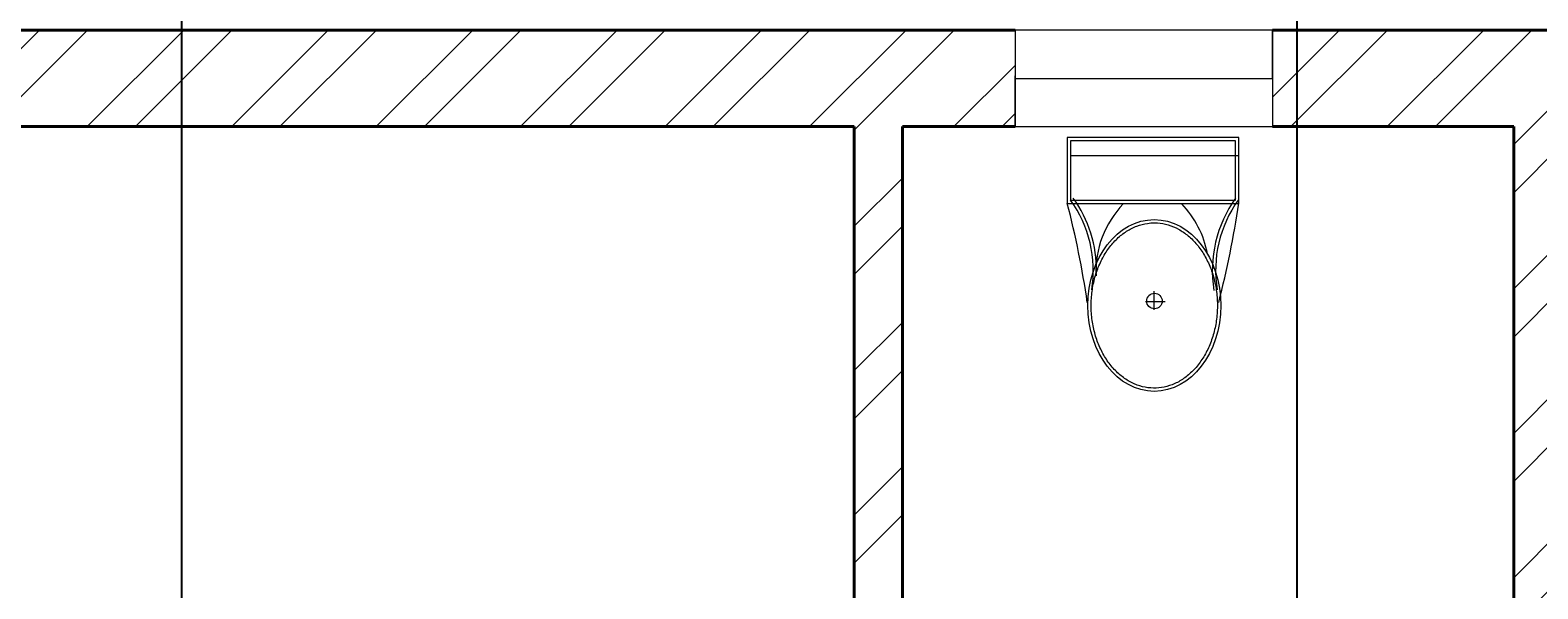
# Model space of a CAD drawing. Units: inches. Extents: x 1601 to 2297, y 1496 to 2631.
# Tile 44 of 57: x 1750 to 1891, y 2480 to 2532. Entities that reach past the tile are written whole.
import ezdxf

# ---------------------------------------------------------------- set-up
doc = ezdxf.new("R2010")
doc.units = ezdxf.units.IN
for name, color, linetype, lineweight in [('A-ANNO-DIMS', 2, 'Continuous', 18), ('A-FLOR-FIXT', 9, 'Continuous', 20), ('A-GLAZ', 161, 'Continuous', 20), ('A-WALL', 7, 'Continuous', 40), ('A-WALL-PATT', 215, 'Continuous', 13)]:
    doc.layers.add(name, color=color, linetype=linetype, lineweight=lineweight)
doc.styles.get("Standard").update_dxf_attribs({"font": 'arial.ttf'})
doc.dimstyles.get("Standard").update_dxf_attribs({"dimtxt": 0.18, "dimasz": 0.18, "dimexe": 0.18, "dimexo": 0.0625, "dimgap": 0.09, "dimtad": 0, "dimtih": 1, "dimtoh": 1, "dimdec": 4, "dimzin": 0, "dimdsep": 46, "dimtxsty": 'Standard', "dimcen": 0.09, "dimadec": 0, "dimazin": 0, "dimtfac": 1, "dimtdec": 4, "dimtofl": 0, "dimtmove": 0, "dimatfit": 3, "dimfxl": 1, "dimtolj": 1, "dimtzin": 0, "dimarcsym": 0})

# ---------------------------------------------------------------- blocks, each defined once
blk = doc.blocks.new('A$C31115884')
for p, q in [((257.5, 466.4), (257.5, 523.2)), ((283.1, 497.7), (223.4, 497.7)), ((0, 200), (0, 0)), ((520, 200), (0, 200)), ((10, 190), (10, 10)), ((510, 190), (10, 190)), ((510, 10), (510, 190)), ((520, 0), (520, 200)), ((510, 54.5), (0, 54.5)), ((10, 10), (510, 10)), ((0, 0), (520, 0))]:
    blk.add_line(p, q)
blk.add_circle((255.6, 496.4), 23.6)
for centre, radius, start, end in [((2777.7, -204.6), 2807, 165.4549, 171.7133), ((-294.5, 403.3), 364.7, 324.2091, 9.3499), ((-294.5, 403.3), 374.7, 324.2091, 9.3499), ((805.8, 403.3), 364.7, 170.6501, 215.7909), ((3237, 905), 2807, 188.2867, 194.5451), ((139.5, 406.2), 293.5, 315.8436, 2.6563), ((805.8, 403.3), 374.7, 179.2036, 215.7909), ((383.6, 406.2), 293.5, 190.2774, 224.1564)]:
    blk.add_arc(centre, radius, start, end)
blk.add_ellipse((256.2, 509.9), major_axis=(0, -260.7), ratio=0.772727)
blk.add_open_spline([(256.2, 259.2), (263.1, 259.2), (270, 259.7), (287.8, 262.3), (298.7, 265.1), (319.9, 273.1), (330.2, 278.4), (350.1, 291.1), (359.7, 298.7), (377.7, 315.9), (386.2, 325.5), (401.7, 346.6), (408.8, 358.1), (421.3, 382.5), (426.8, 395.5), (435.9, 422.4), (439.5, 436.4), (444.8, 465.1), (446.5, 479.7), (447.9, 509.2), (447.6, 524), (445, 553.3), (442.7, 567.8), (436.3, 596), (432.1, 609.7), (421.9, 636), (416, 648.6), (402.5, 672.1), (395, 683), (378.6, 703), (369.8, 712.1), (351.1, 728), (341.3, 734.8), (320.9, 746.2), (310.4, 750.7), (288.9, 757.3), (278, 759.4), (256, 761), (245, 760.6), (223.1, 757.2), (212.3, 754.3), (191.1, 746.1), (180.8, 740.7), (160.9, 727.8), (151.4, 720.1), (133.5, 702.7), (125.1, 693), (109.6, 671.7), (102.6, 660.2), (90.2, 635.7), (84.9, 622.7), (76, 595.6), (72.4, 581.6), (67.2, 552.9), (65.6, 538.2), (64.4, 508.8), (64.8, 494), (67.5, 464.7), (69.9, 450.2), (76.6, 422), (80.8, 408.3), (91.1, 382.2), (97.2, 369.7), (110.8, 346.3), (118.4, 335.4), (134.8, 315.6), (143.7, 306.7), (162.4, 290.9), (172.3, 284.2), (192.8, 273), (203.3, 268.6), (224.8, 262.2), (235.8, 260.2), (249.9, 259.3), (253, 259.2), (256.2, 259.2)], degree=3, knots=[0, 0, 0, 0, 0.110105, 0.110105, 0.285049, 0.285049, 0.459994, 0.459994, 0.634938, 0.634938, 0.809882, 0.809882, 0.984827, 0.984827, 1.159771, 1.159771, 1.334715, 1.334715, 1.50966, 1.50966, 1.684604, 1.684604, 1.859549, 1.859549, 2.034493, 2.034493, 2.209437, 2.209437, 2.384382, 2.384382, 2.559326, 2.559326, 2.73427, 2.73427, 2.909215, 2.909215, 3.084159, 3.084159, 3.259103, 3.259103, 3.434048, 3.434048, 3.608992, 3.608992, 3.783936, 3.783936, 3.958881, 3.958881, 4.133825, 4.133825, 4.30877, 4.30877, 4.483714, 4.483714, 4.658658, 4.658658, 4.833603, 4.833603, 5.008547, 5.008547, 5.183491, 5.183491, 5.358436, 5.358436, 5.53338, 5.53338, 5.708324, 5.708324, 5.883269, 5.883269, 6.058213, 6.058213, 6.233158, 6.233158, 6.283185, 6.283185, 6.283185, 6.283185])
blk = doc.blocks.new('*D33')
at = {"layer": 'A-ANNO-DIMS', "color": 0, "lineweight": -2, "transparency": 16777216}
for p, q in [((1764.34, 2136.39), (1764.34, 2581.06)), ((1764.52, 2580.88), (1816.06, 2580.88)), ((1868.16, 2580.88), (1816.62, 2580.88)), ((1868.34, 2136.39), (1868.34, 2581.06))]:
    blk.add_line(p, q, dxfattribs=at)
at = {"layer": 'A-ANNO-DIMS', "color": 0, "transparency": 16777216}
for points in [[(1764.52, 2580.91), (1764.52, 2580.85), (1764.34, 2580.88)], [(1868.16, 2580.91), (1868.16, 2580.85), (1868.34, 2580.88)]]:
    blk.add_solid(points, dxfattribs=at)
at = {"layer": 'Defpoints', "color": 0, "transparency": 16777216}
for p in [(1868.34, 2580.88), (1764.34, 2136.33), (1868.34, 2136.33)]:
    blk.add_point(p, dxfattribs=at)
at = {"layer": 'A-ANNO-DIMS', "color": 0, "transparency": 16777216, "insert": (1816.34, 2580.88), "char_height": 0.18, "attachment_point": 5}
blk.add_mtext('\\A1;104', dxfattribs=at)

msp = doc.modelspace()

# ---------------------------------------------------------------- hatches: boundary and pattern name
at = {"layer": 'A-WALL-PATT'}
h = msp.add_hatch(dxfattribs=at)
h.set_pattern_fill('ANSI32', color=256)
h.paths.add_polyline_path([(1842.0336, 2528.0767), (1842.0336, 2532.3254), (1686.0373, 2532.3254), (1686.0373, 2492.9493), (1695.0373, 2492.9493), (1695.0373, 2523.3254), (1827.0373, 2523.3254), (1827.0373, 2416.8254), (1834.6225, 2416.8254), (1834.6225, 2419.0754), (1834.6225, 2421.3254), (1831.5373, 2421.3254), (1831.5373, 2523.3254), (1842.0336, 2523.3254)])
h.paths.add_polyline_path([(1695.0373, 2432.9493), (1686.0373, 2432.9493), (1686.0373, 2325.989), (1695.0373, 2325.989), (1695.0373, 2347.8254), (1827.0373, 2347.8254), (1827.0373, 2287.8254), (1823.2991, 2287.8254), (1823.2991, 2283.3254), (1847.9422, 2283.3254), (1847.9422, 2285.5754), (1847.9422, 2287.8254), (1831.5373, 2287.8254), (1831.5373, 2347.8254), (1846.9946, 2347.8254), (1846.9946, 2350.0754), (1846.9946, 2352.3254), (1695.0373, 2352.3254)])
h.paths.add_polyline_path([(1807.1169, 1573.5395), (2055.0405, 1573.5395), (2055.0405, 1610.6322), (1807.1169, 1610.6322)], flags=9)
h.paths.add_polyline_path([(1841.1631, 1712.7967), (1870.3957, 1712.7967), (1870.3957, 1731.454), (1841.1631, 1731.454)], flags=9)
h.paths.add_polyline_path([(2144.3862, 1772.185), (2191.0233, 1772.185), (2191.0233, 1790.8423), (2144.3862, 1790.8423)], flags=9)
h.paths.add_polyline_path([(2143.0128, 1827.3312), (2177.9958, 1827.3312), (2177.9958, 1845.9886), (2143.0128, 1845.9886)], flags=9)
h.paths.add_polyline_path([(2041.2439, 1833.5691), (2070.8516, 1833.5691), (2070.8516, 1852.2264), (2041.2439, 1852.2264)], flags=9)
h.paths.add_polyline_path([(2097.2791, 1947.0598), (2134.2061, 1947.0598), (2134.2061, 1965.7171), (2097.2791, 1965.7171)], flags=9)
h.paths.add_polyline_path([(2214.995, 1904.3124), (2214.995, 1942.2899), (2196.3376, 1942.2899), (2196.3376, 1904.3124)], flags=9)
h.paths.add_polyline_path([(2186.6284, 2043.8031), (2219.7935, 2043.8031), (2219.7935, 2062.4605), (2186.6284, 2062.4605)], flags=9)
h.paths.add_polyline_path([(2064.0877, 2031.616), (2097.4949, 2031.616), (2097.4949, 2050.2734), (2064.0877, 2050.2734)], flags=9)
h.paths.add_polyline_path([(1973.1349, 1986.0688), (2008.4009, 1986.0688), (2008.4009, 2004.7261), (1973.1349, 2004.7261)], flags=9)
h.paths.add_polyline_path([(1976.3676, 2106.9635), (2005.7469, 2106.9635), (2005.7469, 2125.6209), (1976.3676, 2125.6209)], flags=9)
h.paths.add_polyline_path([(1991.7852, 2180.4863), (2027.0513, 2180.4863), (2027.0513, 2199.1437), (1991.7852, 2199.1437)], flags=9)
h.paths.add_polyline_path([(2106.1801, 2187.9359), (2152.2101, 2187.9359), (2152.2101, 2206.5932), (2106.1801, 2206.5932)], flags=9)
h.paths.add_polyline_path([(2148.6686, 2262.2542), (2182.318, 2262.2542), (2182.318, 2280.9115), (2148.6686, 2280.9115)], flags=9)
h.paths.add_polyline_path([(2041.6327, 2252.8147), (2071.2405, 2252.8147), (2071.2405, 2271.4721), (2041.6327, 2271.4721)], flags=9)
h.paths.add_polyline_path([(2063.9734, 2375.4265), (2100.9004, 2375.4265), (2100.9004, 2394.0839), (2063.9734, 2394.0839)], flags=9)
h.paths.add_polyline_path([(2216.4955, 2330.9748), (2216.4955, 2370.2654), (2197.8381, 2370.2654), (2197.8381, 2330.9748)], flags=9)
h.paths.add_polyline_path([(2179.1416, 2485.8687), (2212.3067, 2485.8687), (2212.3067, 2504.5261), (2179.1416, 2504.5261)], flags=9)
h.paths.add_polyline_path([(2078.7442, 2471.1516), (2112.1514, 2471.1516), (2112.1514, 2489.809), (2078.7442, 2489.809)], flags=9)
h.paths.add_polyline_path([(1915.9631, 2329.4668), (1952.8902, 2329.4668), (1952.8902, 2348.1241), (1915.9631, 2348.1241)], flags=9)
h.paths.add_polyline_path([(1904.3189, 2499.6709), (1940.4512, 2499.6709), (1940.4512, 2518.3282), (1904.3189, 2518.3282)], flags=9)
h.paths.add_polyline_path([(1892.3665, 2100.4595), (1925.6374, 2100.4595), (1925.6374, 2119.1169), (1892.3665, 2119.1169)], flags=9)
h.paths.add_polyline_path([(1909.2984, 1805.9631), (1946.2254, 1805.9631), (1946.2254, 1824.6205), (1909.2984, 1824.6205)], flags=9)
h.paths.add_polyline_path([(1934.6056, 1658.616), (1970.738, 1658.616), (1970.738, 1677.2733), (1934.6056, 1677.2733)], flags=9)
h.paths.add_polyline_path([(1711.2052, 1789.8902), (1750.0456, 1789.8902), (1750.0456, 1808.5476), (1711.2052, 1808.5476)], flags=9)
h.paths.add_polyline_path([(1742.7874, 1854.6743), (1771.9449, 1854.6743), (1771.9449, 1873.3317), (1742.7874, 1873.3317)], flags=9)
h.paths.add_polyline_path([(1807.3592, 1997.7912), (1850.1116, 1997.7912), (1850.1116, 2016.4486), (1807.3592, 2016.4486)], flags=9)
h.paths.add_polyline_path([(1717.4579, 2237.7844), (1760.2103, 2237.7844), (1760.2103, 2256.4417), (1717.4579, 2256.4417)], flags=9)
h.paths.add_polyline_path([(1780.9285, 2324.0623), (1810.086, 2324.0623), (1810.086, 2342.7197), (1780.9285, 2342.7197)], flags=25)
h.paths.add_polyline_path([(1837.696, 2449.2024), (1866.9286, 2449.2024), (1866.9286, 2467.8598), (1837.696, 2467.8598)], flags=9)
h.paths.add_polyline_path([(1712.7752, 2484.9404), (1751.6156, 2484.9404), (1751.6156, 2503.5977), (1712.7752, 2503.5977)], flags=25)
h = msp.add_hatch(dxfattribs=at)
h.set_pattern_fill('ANSI32', color=256)
h.paths.add_polyline_path([(2230.5373, 2532.3254), (2106.0595, 2532.3254), (2106.0595, 2523.3254), (2169.0373, 2523.3254), (2169.0373, 2424.3254), (2091.3989, 2424.3254), (2091.3989, 2419.8254), (2169.0373, 2419.8254), (2169.0373, 2408.1385), (2178.0373, 2408.1385), (2178.0373, 2419.8254), (2181.0581, 2419.8254), (2181.0581, 2422.0754), (2181.0581, 2424.3254), (2178.0373, 2424.3254), (2178.0373, 2523.3254), (2226.0373, 2523.3254), (2226.0373, 2424.3254), (2206.6251, 2424.3254), (2206.6251, 2419.8254), (2226.0373, 2419.8254), (2226.0373, 2299.8254), (2226.0373, 2295.3254), (2178.0373, 2295.3254), (2178.0373, 2312.1385), (2169.0373, 2312.1385), (2169.0373, 2295.3254), (2130.0373, 2295.3254), (2130.0373, 2279.1364), (2128.0593, 2279.1364), (2128.0593, 2274.6364), (2130.0373, 2274.6364), (2130.0373, 2260.7505), (2134.5373, 2260.7505), (2134.5373, 2290.8254), (2226.0373, 2290.8254), (2226.0373, 2279.2475), (2230.5373, 2279.2475), (2230.5373, 2347.8254)])
h.paths.add_polyline_path([(2070.0595, 2532.3254), (2031.0373, 2532.3254), (2031.0373, 2466.3254), (2003.9878, 2466.3254), (2003.9878, 2457.3254), (2031.0373, 2457.3254), (2031.0373, 2419.8254), (2031.0373, 2373.1914), (2035.5373, 2373.1914), (2035.5373, 2419.8254), (2047.3393, 2419.8254), (2047.3393, 2424.3254), (2035.5373, 2424.3254), (2035.5373, 2523.3254), (2070.0595, 2523.3254), (2070.0595, 2527.8254)])
h.paths.add_polyline_path([(1893.0373, 2532.3254), (1866.0336, 2532.3254), (1866.0336, 2523.3254), (1888.5373, 2523.3254), (1888.5373, 2347.8254), (1893.0373, 2347.8254), (1893.0373, 2457.3254), (1907.9878, 2457.3254), (1907.9878, 2466.3254), (1893.0373, 2466.3254)])
h = msp.add_hatch(dxfattribs=at)
h.set_pattern_fill('ANSI32', color=256)
h.paths.add_polyline_path([(1973.9371, 2211.3254), (1893.0373, 2211.3254), (1893.0373, 2287.8254), (1884.6167, 2287.8254), (1884.6167, 2285.5754), (1884.6167, 2283.3254), (1888.5373, 2283.3254), (1888.5373, 2145.3254), (1695.0373, 2145.3254), (1695.0373, 2173.8724), (1690.5373, 2173.8724), (1686.0373, 2173.8724), (1686.0373, 2136.3254), (1722.5687, 2136.3254), (1722.5687, 2117.4352), (1731.5687, 2117.4352), (1731.5687, 2136.3254), (1893.0373, 2136.3254), (1893.0373, 2202.3254), (1959.0373, 2202.3254), (1959.0373, 2182.1303), (1968.0373, 2182.1303), (1968.0373, 2202.3254), (1973.9371, 2202.3254)])
h.paths.add_polyline_path([(2094.0373, 2274.6364), (2096.4294, 2274.6364), (2096.4294, 2276.8864), (2096.4294, 2279.1364), (2094.0373, 2279.1364), (2094.0373, 2290.8254), (2094.0373, 2295.3254), (2089.5373, 2295.3254), (2089.5373, 2230.8254), (2035.5373, 2230.8254), (2035.5373, 2299.8254), (2031.0373, 2299.8254), (2031.0373, 2211.3254), (2023.0065, 2211.3254), (2023.0065, 2202.3254), (2031.0373, 2202.3254), (2031.0373, 2140.8254), (1968.0373, 2140.8254), (1968.0373, 2145.9106), (1963.5373, 2145.9106), (1959.0373, 2145.9106), (1959.0373, 2116.839), (1963.5373, 2116.839), (1968.0373, 2116.839), (1968.0373, 2131.8254), (2031.0373, 2131.8254), (2031.0373, 2094.3254), (2031.0373, 2085.3254), (2031.0373, 2056.8254), (1968.0373, 2056.8254), (1968.0373, 2070.4947), (1963.5373, 2070.4947), (1959.0373, 2070.4947), (1959.0373, 2040.3029), (1968.0373, 2040.3029), (1968.0373, 2047.8254), (2031.0373, 2047.8254), (2031.0373, 1983.3254), (2031.0373, 1978.8254), (2021.1979, 1978.8254), (2021.1979, 1974.3254), (2031.0373, 1974.3254), (2031.0373, 1954.3528), (2035.5373, 1954.3528), (2035.5373, 1974.3254), (2035.5373, 1981.8254), (2055.5513, 1981.8254), (2055.5513, 1986.3254), (2035.5373, 1986.3254), (2035.5373, 2047.8254), (2040.0373, 2047.8254), (2040.0373, 2085.3254), (2040.0373, 2094.3254), (2040.0373, 2140.8254), (2035.5373, 2140.8254), (2035.5373, 2226.3254), (2089.5373, 2226.3254), (2094.0373, 2226.3254)])
h.paths.add_polyline_path([(2226.0373, 2230.8254), (2134.5373, 2230.8254), (2134.5373, 2233.5437), (2130.0373, 2233.5437), (2130.0373, 2226.3254), (2134.5373, 2226.3254), (2226.0373, 2226.3254)])
h.paths.add_polyline_path([(1807.1169, 1573.5395), (2055.0405, 1573.5395), (2055.0405, 1610.6322), (1807.1169, 1610.6322)], flags=9)
h.paths.add_polyline_path([(1841.1631, 1712.7967), (1870.3957, 1712.7967), (1870.3957, 1731.454), (1841.1631, 1731.454)], flags=9)
h.paths.add_polyline_path([(2144.3862, 1772.185), (2191.0233, 1772.185), (2191.0233, 1790.8423), (2144.3862, 1790.8423)], flags=9)
h.paths.add_polyline_path([(2143.0128, 1827.3312), (2177.9958, 1827.3312), (2177.9958, 1845.9886), (2143.0128, 1845.9886)], flags=9)
h.paths.add_polyline_path([(2041.2439, 1833.5691), (2070.8516, 1833.5691), (2070.8516, 1852.2264), (2041.2439, 1852.2264)], flags=9)
h.paths.add_polyline_path([(2097.2791, 1947.0598), (2134.2061, 1947.0598), (2134.2061, 1965.7171), (2097.2791, 1965.7171)], flags=9)
h.paths.add_polyline_path([(2214.995, 1904.3124), (2214.995, 1942.2899), (2196.3376, 1942.2899), (2196.3376, 1904.3124)], flags=9)
h.paths.add_polyline_path([(2186.6284, 2043.8031), (2219.7935, 2043.8031), (2219.7935, 2062.4605), (2186.6284, 2062.4605)], flags=9)
h.paths.add_polyline_path([(2064.0877, 2031.616), (2097.4949, 2031.616), (2097.4949, 2050.2734), (2064.0877, 2050.2734)], flags=9)
h.paths.add_polyline_path([(1973.1349, 1986.0688), (2008.4009, 1986.0688), (2008.4009, 2004.7261), (1973.1349, 2004.7261)], flags=25)
h.paths.add_polyline_path([(1976.3676, 2106.9635), (2005.7469, 2106.9635), (2005.7469, 2125.6209), (1976.3676, 2125.6209)], flags=25)
h.paths.add_polyline_path([(1991.7852, 2180.4863), (2027.0513, 2180.4863), (2027.0513, 2199.1437), (1991.7852, 2199.1437)], flags=25)
h.paths.add_polyline_path([(2106.1801, 2187.9359), (2152.2101, 2187.9359), (2152.2101, 2206.5932), (2106.1801, 2206.5932)], flags=9)
h.paths.add_polyline_path([(2148.6686, 2262.2542), (2182.318, 2262.2542), (2182.318, 2280.9115), (2148.6686, 2280.9115)], flags=9)
h.paths.add_polyline_path([(2041.6327, 2252.8147), (2071.2405, 2252.8147), (2071.2405, 2271.4721), (2041.6327, 2271.4721)], flags=25)
h.paths.add_polyline_path([(2063.9734, 2375.4265), (2100.9004, 2375.4265), (2100.9004, 2394.0839), (2063.9734, 2394.0839)], flags=9)
h.paths.add_polyline_path([(2216.4955, 2330.9748), (2216.4955, 2370.2654), (2197.8381, 2370.2654), (2197.8381, 2330.9748)], flags=9)
h.paths.add_polyline_path([(2179.1416, 2485.8687), (2212.3067, 2485.8687), (2212.3067, 2504.5261), (2179.1416, 2504.5261)], flags=9)
h.paths.add_polyline_path([(2078.7442, 2471.1516), (2112.1514, 2471.1516), (2112.1514, 2489.809), (2078.7442, 2489.809)], flags=9)
h.paths.add_polyline_path([(1915.9631, 2329.4668), (1952.8902, 2329.4668), (1952.8902, 2348.1241), (1915.9631, 2348.1241)], flags=9)
h.paths.add_polyline_path([(1904.3189, 2499.6709), (1940.4512, 2499.6709), (1940.4512, 2518.3282), (1904.3189, 2518.3282)], flags=9)
h.paths.add_polyline_path([(1892.3665, 2100.4595), (1925.6374, 2100.4595), (1925.6374, 2119.1169), (1892.3665, 2119.1169)], flags=9)
h.paths.add_polyline_path([(1909.2984, 1805.9631), (1946.2254, 1805.9631), (1946.2254, 1824.6205), (1909.2984, 1824.6205)], flags=9)
h.paths.add_polyline_path([(1934.6056, 1658.616), (1970.738, 1658.616), (1970.738, 1677.2733), (1934.6056, 1677.2733)], flags=9)
h.paths.add_polyline_path([(1711.2052, 1789.8902), (1750.0456, 1789.8902), (1750.0456, 1808.5476), (1711.2052, 1808.5476)], flags=9)
h.paths.add_polyline_path([(1742.7874, 1854.6743), (1771.9449, 1854.6743), (1771.9449, 1873.3317), (1742.7874, 1873.3317)], flags=9)
h.paths.add_polyline_path([(1807.3592, 1997.7912), (1850.1116, 1997.7912), (1850.1116, 2016.4486), (1807.3592, 2016.4486)], flags=9)
h.paths.add_polyline_path([(1717.4579, 2237.7844), (1760.2103, 2237.7844), (1760.2103, 2256.4417), (1717.4579, 2256.4417)], flags=25)
h.paths.add_polyline_path([(1780.9285, 2324.0623), (1810.086, 2324.0623), (1810.086, 2342.7197), (1780.9285, 2342.7197)], flags=9)
h.paths.add_polyline_path([(1837.696, 2449.2024), (1866.9286, 2449.2024), (1866.9286, 2467.8598), (1837.696, 2467.8598)], flags=9)
h.paths.add_polyline_path([(1712.7752, 2484.9404), (1751.6156, 2484.9404), (1751.6156, 2503.5977), (1712.7752, 2503.5977)], flags=9)
h = msp.add_hatch(dxfattribs=at)
h.set_pattern_fill('ANSI32', color=256)
h.paths.add_polyline_path([(2230.5373, 1861.8254), (2182.5373, 1861.8254), (2182.5373, 1885.3637), (2178.0373, 1885.3637), (2178.0373, 1861.8254), (2166.0373, 1861.8254), (2134.5373, 1861.8254), (2130.0373, 1861.8254), (2130.0373, 1841.4682), (2126.8833, 1841.4682), (2126.8833, 1836.9682), (2130.0373, 1836.9682), (2130.0373, 1822.7302), (2134.5373, 1822.7302), (2134.5373, 1857.3254), (2166.0373, 1857.3254), (2226.0373, 1857.3254), (2226.0373, 1846.1155), (2230.5373, 1846.1155)])
h.paths.add_polyline_path([(2226.0373, 1797.3254), (2134.5373, 1797.3254), (2134.5373, 1800.6636), (2132.2873, 1800.6636), (2130.0373, 1800.6636), (2130.0373, 1797.3254), (2130.0373, 1792.8254), (2167.7264, 1792.8254), (2226.0373, 1792.8254)])
h.paths.add_polyline_path([(2230.5373, 1822.1155), (2226.0373, 1822.1155), (2226.0373, 1760.8563), (2230.5373, 1760.8563)])
h.paths.add_polyline_path([(2230.5373, 1700.8563), (2226.0373, 1700.8563), (2226.0373, 1644.3254), (2140.2517, 1644.3254), (2140.2517, 1635.3254), (2230.5373, 1635.3254)])
h.paths.add_polyline_path([(2080.2517, 1639.8254), (2080.2517, 1644.3254), (2035.5373, 1644.3254), (2035.5373, 1792.8254), (2094.0373, 1792.8254), (2094.0373, 1797.3254), (2094.0373, 1836.9682), (2097.1057, 1836.9682), (2097.1057, 1839.2182), (2097.1057, 1841.4682), (2094.0373, 1841.4682), (2094.0373, 1862.2276), (2089.5373, 1862.2276), (2089.5373, 1797.3254), (2035.5373, 1797.3254), (2035.5373, 1857.3254), (2035.5373, 1885.0916), (2031.0373, 1885.0916), (2031.0373, 1710.3254), (2012.329, 1710.3254), (2012.329, 1701.3254), (2031.0373, 1701.3254), (2031.0373, 1644.3254), (2031.0373, 1635.3254), (2080.2517, 1635.3254)])
h.paths.add_polyline_path([(1836.0373, 1653.2033), (1842.6171, 1653.2033), (1842.6171, 1657.7033), (1842.6171, 1662.2033), (1831.5373, 1662.2033), (1831.5373, 1764.2033), (1835.3881, 1764.2033), (1835.3881, 1766.4533), (1835.3881, 1768.7033), (1831.5373, 1768.7033), (1827.0373, 1768.7033), (1827.0373, 1662.2033), (1827.0373, 1635.3254), (1836.0373, 1635.3254)])
h.paths.add_polyline_path([(1893.0373, 1701.3254), (1907.193, 1701.3254), (1907.193, 1705.8254), (1907.193, 1710.3254), (1893.0373, 1710.3254), (1893.0373, 1819.8254), (1882.6444, 1819.8254), (1882.6444, 1817.5754), (1882.6444, 1815.3254), (1888.5373, 1815.3254), (1888.5373, 1662.2033), (1884.0373, 1662.2033), (1866.6171, 1662.2033), (1866.6171, 1653.2033), (1882.391, 1653.2033), (1884.0373, 1653.2033), (1884.0373, 1635.3254), (1893.0373, 1635.3254)])
h.paths.add_polyline_path([(1739.3335, 1639.8254), (1739.3335, 1644.3254), (1695.0373, 1644.3254), (1695.0373, 1702.0135), (1690.5373, 1702.0135), (1686.0373, 1702.0135), (1686.0373, 1635.3254), (1739.3335, 1635.3254)])
h.paths.add_polyline_path([(1827.0373, 1644.3254), (1799.3335, 1644.3254), (1799.3335, 1635.3254), (1827.0373, 1635.3254)])
h.paths.add_polyline_path([(1695.0373, 1815.3254), (1849.2759, 1815.3254), (1849.2759, 1819.8254), (1807.5373, 1819.8254), (1807.5373, 1879.8254), (1851.1533, 1879.8254), (1851.1533, 1882.0754), (1851.1533, 1884.3254), (1799.3405, 1884.3254), (1799.3405, 1882.0754), (1799.3405, 1879.8254), (1803.0373, 1879.8254), (1803.0373, 1819.8254), (1695.0373, 1819.8254), (1695.0373, 1835.0458), (1690.5373, 1835.0458), (1686.0373, 1835.0458), (1686.0373, 1766.1753), (1695.0373, 1766.1753)])
h.paths.add_polyline_path([(1775.8157, 1884.3254), (1695.0373, 1884.3254), (1695.0373, 1912.9526), (1690.5373, 1912.9526), (1686.0373, 1912.9526), (1686.0373, 1859.0458), (1695.0373, 1859.0458), (1695.0373, 1879.8254), (1775.8157, 1879.8254)])
h.paths.add_polyline_path([(1893.0373, 2031.3254), (1731.5687, 2031.3254), (1731.5687, 2057.4352), (1722.5687, 2057.4352), (1722.5687, 2031.3254), (1686.0373, 2031.3254), (1686.0373, 1972.9526), (1695.0373, 1972.9526), (1695.0373, 2022.3254), (1888.5373, 2022.3254), (1888.5373, 1884.3254), (1883.4996, 1884.3254), (1883.4996, 1879.8254), (1893.0373, 1879.8254), (1893.0373, 1974.3254), (1976.6199, 1974.3254), (1976.6199, 1978.8254), (1968.0373, 1978.8254), (1968.0373, 1983.3254), (1968.0373, 2008.4756), (1963.5373, 2008.4756), (1959.0373, 2008.4756), (1959.0373, 1983.3254), (1893.0373, 1983.3254)])
h.paths.add_polyline_path([(2230.5373, 2140.4745), (2226.0373, 2140.4745), (2226.0373, 2094.3254), (2040.0373, 2094.3254), (2040.0373, 2085.3254), (2178.0373, 2085.3254), (2178.0373, 2065.6965), (2182.5373, 2065.6965), (2182.5373, 2085.3254), (2226.0373, 2085.3254), (2226.0373, 1986.3254), (2211.2679, 1986.3254), (2211.2679, 1981.8254), (2230.5373, 1981.8254)])
h.paths.add_polyline_path([(2187.6292, 1986.3254), (2182.5373, 1986.3254), (2182.5373, 2029.6965), (2178.0373, 2029.6965), (2178.0373, 1986.3254), (2099.05, 1986.3254), (2099.05, 1981.8254), (2178.0373, 1981.8254), (2178.0373, 1969.3637), (2182.5373, 1969.3637), (2182.5373, 1981.8254), (2187.6292, 1981.8254), (2187.6292, 1984.0754)])
h.paths.add_polyline_path([(1807.1169, 1573.5395), (2055.0405, 1573.5395), (2055.0405, 1610.6322), (1807.1169, 1610.6322)], flags=9)
h.paths.add_polyline_path([(1841.1631, 1712.7967), (1870.3957, 1712.7967), (1870.3957, 1731.454), (1841.1631, 1731.454)], flags=9)
h.paths.add_polyline_path([(2144.3862, 1772.185), (2191.0233, 1772.185), (2191.0233, 1790.8423), (2144.3862, 1790.8423)], flags=9)
h.paths.add_polyline_path([(2143.0128, 1827.3312), (2177.9958, 1827.3312), (2177.9958, 1845.9886), (2143.0128, 1845.9886)], flags=25)
h.paths.add_polyline_path([(2041.2439, 1833.5691), (2070.8516, 1833.5691), (2070.8516, 1852.2264), (2041.2439, 1852.2264)], flags=25)
h.paths.add_polyline_path([(2097.2791, 1947.0598), (2134.2061, 1947.0598), (2134.2061, 1965.7171), (2097.2791, 1965.7171)], flags=9)
h.paths.add_polyline_path([(2214.995, 1904.3124), (2214.995, 1942.2899), (2196.3376, 1942.2899), (2196.3376, 1904.3124)], flags=9)
h.paths.add_polyline_path([(2186.6284, 2043.8031), (2219.7935, 2043.8031), (2219.7935, 2062.4605), (2186.6284, 2062.4605)], flags=25)
h.paths.add_polyline_path([(2064.0877, 2031.616), (2097.4949, 2031.616), (2097.4949, 2050.2734), (2064.0877, 2050.2734)], flags=25)
h.paths.add_polyline_path([(1973.1349, 1986.0688), (2008.4009, 1986.0688), (2008.4009, 2004.7261), (1973.1349, 2004.7261)], flags=9)
h.paths.add_polyline_path([(1976.3676, 2106.9635), (2005.7469, 2106.9635), (2005.7469, 2125.6209), (1976.3676, 2125.6209)], flags=9)
h.paths.add_polyline_path([(1991.7852, 2180.4863), (2027.0513, 2180.4863), (2027.0513, 2199.1437), (1991.7852, 2199.1437)], flags=9)
h.paths.add_polyline_path([(2106.1801, 2187.9359), (2152.2101, 2187.9359), (2152.2101, 2206.5932), (2106.1801, 2206.5932)], flags=9)
h.paths.add_polyline_path([(2148.6686, 2262.2542), (2182.318, 2262.2542), (2182.318, 2280.9115), (2148.6686, 2280.9115)], flags=9)
h.paths.add_polyline_path([(2041.6327, 2252.8147), (2071.2405, 2252.8147), (2071.2405, 2271.4721), (2041.6327, 2271.4721)], flags=9)
h.paths.add_polyline_path([(2063.9734, 2375.4265), (2100.9004, 2375.4265), (2100.9004, 2394.0839), (2063.9734, 2394.0839)], flags=9)
h.paths.add_polyline_path([(2216.4955, 2330.9748), (2216.4955, 2370.2654), (2197.8381, 2370.2654), (2197.8381, 2330.9748)], flags=9)
h.paths.add_polyline_path([(2179.1416, 2485.8687), (2212.3067, 2485.8687), (2212.3067, 2504.5261), (2179.1416, 2504.5261)], flags=9)
h.paths.add_polyline_path([(2078.7442, 2471.1516), (2112.1514, 2471.1516), (2112.1514, 2489.809), (2078.7442, 2489.809)], flags=9)
h.paths.add_polyline_path([(1915.9631, 2329.4668), (1952.8902, 2329.4668), (1952.8902, 2348.1241), (1915.9631, 2348.1241)], flags=9)
h.paths.add_polyline_path([(1904.3189, 2499.6709), (1940.4512, 2499.6709), (1940.4512, 2518.3282), (1904.3189, 2518.3282)], flags=9)
h.paths.add_polyline_path([(1892.3665, 2100.4595), (1925.6374, 2100.4595), (1925.6374, 2119.1169), (1892.3665, 2119.1169)], flags=9)
h.paths.add_polyline_path([(1909.2984, 1805.9631), (1946.2254, 1805.9631), (1946.2254, 1824.6205), (1909.2984, 1824.6205)], flags=9)
h.paths.add_polyline_path([(1934.6056, 1658.616), (1970.738, 1658.616), (1970.738, 1677.2733), (1934.6056, 1677.2733)], flags=9)
h.paths.add_polyline_path([(1711.2052, 1789.8902), (1750.0456, 1789.8902), (1750.0456, 1808.5476), (1711.2052, 1808.5476)], flags=25)
h.paths.add_polyline_path([(1742.7874, 1854.6743), (1771.9449, 1854.6743), (1771.9449, 1873.3317), (1742.7874, 1873.3317)], flags=25)
h.paths.add_polyline_path([(1807.3592, 1997.7912), (1850.1116, 1997.7912), (1850.1116, 2016.4486), (1807.3592, 2016.4486)], flags=25)
h.paths.add_polyline_path([(1717.4579, 2237.7844), (1760.2103, 2237.7844), (1760.2103, 2256.4417), (1717.4579, 2256.4417)], flags=9)
h.paths.add_polyline_path([(1780.9285, 2324.0623), (1810.086, 2324.0623), (1810.086, 2342.7197), (1780.9285, 2342.7197)], flags=9)
h.paths.add_polyline_path([(1837.696, 2449.2024), (1866.9286, 2449.2024), (1866.9286, 2467.8598), (1837.696, 2467.8598)], flags=9)
h.paths.add_polyline_path([(1712.7752, 2484.9404), (1751.6156, 2484.9404), (1751.6156, 2503.5977), (1712.7752, 2503.5977)], flags=9)

# ---------------------------------------------------------------- linework, layer by layer
at = {"layer": 'A-GLAZ'}
for p, q in [((1842.0336, 2532.3254), (1842.0336, 2523.3254)), ((1866.0336, 2532.3254), (1842.0336, 2532.3254)), ((1866.0336, 2527.8254), (1866.0336, 2532.3254)), ((1866.0336, 2532.3254), (1866.0336, 2523.3254)), ((1842.0336, 2523.3254), (1842.0336, 2528.0767)), ((1842.0336, 2528.0767), (1842.0336, 2527.8254)), ((1842.0336, 2527.8254), (1866.0336, 2527.8254)), ((1842.0336, 2523.3254), (1866.0336, 2523.3254))]:
    msp.add_line(p, q, dxfattribs=at)
at = {"layer": 'A-WALL'}
for p, q in [((1686.0373, 2532.3254), (1842.0336, 2532.3254)), ((1866.0336, 2532.3254), (2070.0595, 2532.3254)), ((1695.0373, 2523.3254), (1827.0373, 2523.3254)), ((1827.0373, 2523.3254), (1827.0373, 2416.8254)), ((1831.5373, 2523.3254), (1831.5373, 2421.3254)), ((1831.5373, 2523.3254), (1842.0336, 2523.3254)), ((1866.0336, 2523.3254), (1888.5373, 2523.3254)), ((1888.5373, 2523.3254), (1888.5373, 2347.8254))]:
    msp.add_line(p, q, dxfattribs=at)

# ---------------------------------------------------------------- block references
at = {"layer": 'A-FLOR-FIXT', "xscale": 0.0307498789965588, "yscale": 0.0307498789965588, "zscale": 0.0307498789965588, "rotation": 180}
msp.add_blockref('A$C31115884', (1862.894, 2522.3164), dxfattribs=at)

# ---------------------------------------------------------------- dimensions: what is measured, and where the dimension line sits
at = {"layer": 'A-ANNO-DIMS'}
dim = msp.add_linear_dim(base=(1868.3371, 2580.8754), p1=(1764.3371, 2136.3254), p2=(1868.3371, 2136.3254), dimstyle='Standard', override={"dimdec": 0, "dimlfac": 1, "dimrnd": 0, "dimzin": 0, "dimdsep": 46, "dimlunit": 2}, dxfattribs=at)
dim.commit()
dim.dimension.update_dxf_attribs({"geometry": '*D33', "text_midpoint": (1816.3371, 2580.8754)})

doc.saveas('drawing.dxf')
